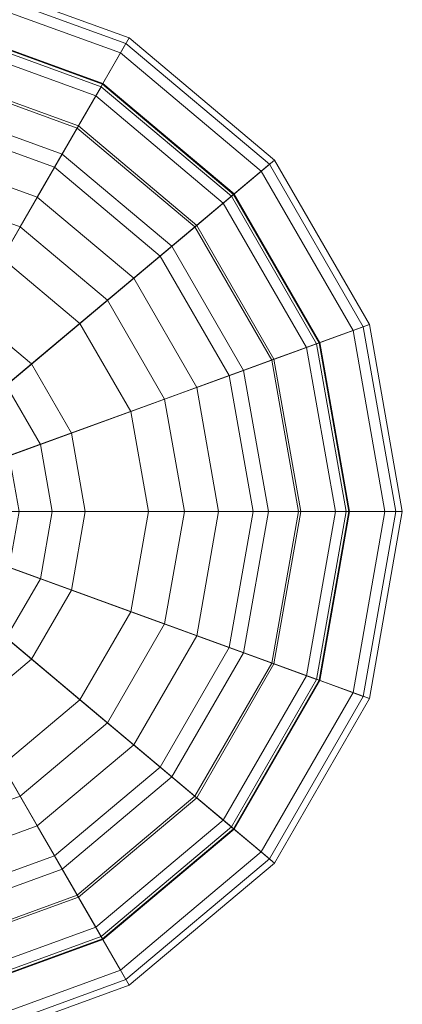
# Model space of a CAD drawing. Units: inches. Extents: x 375 to 1122, y 27 to 1069.
# Tile 43 of 155: x 719.669 to 720.617, y 297.867 to 300.305. Entities that reach past the tile are written whole.
import ezdxf

# ---------------------------------------------------------------- set-up
doc = ezdxf.new("R2010")
doc.units = ezdxf.units.IN
doc.layers.add('Furniture', color=30, linetype='Continuous', lineweight=18)

# ---------------------------------------------------------------- blocks, each defined once
blk = doc.blocks.new('A$C403C54AD')
for points in [[(1.180252, 0.891746, -0.031825), (1.180252, 0.857884, -0.028747), (1.180252, 0.857884, -0.028747), (1.16867, 0.889704, -0.031825)], [(1.180252, 0.88848, -0.028594), (1.180252, 0.891746, -0.031825), (1.16867, 0.889704, -0.031825), (1.169787, 0.886635, -0.028594)], [(1.191834, 0.889704, -0.031825), (1.180252, 0.857884, -0.028747), (1.180252, 0.857884, -0.028747), (1.180252, 0.891746, -0.031825)], [(1.190717, 0.886635, -0.028594), (1.191834, 0.889704, -0.031825), (1.180252, 0.891746, -0.031825), (1.180252, 0.88848, -0.028594)], [(1.180252, 0.88844, 0.131159), (1.180252, 0.891347, 0.117935), (1.168807, 0.889329, 0.117935), (1.169801, 0.886597, 0.131159)], [(1.180252, 0.891347, 0.117935), (1.180252, 0.890672, 0.089693), (1.169038, 0.888695, 0.089693), (1.168807, 0.889329, 0.117935)], [(1.190703, 0.886597, 0.131159), (1.191697, 0.889329, 0.117935), (1.180252, 0.891347, 0.117935), (1.180252, 0.88844, 0.131159)], [(1.191697, 0.889329, 0.117935), (1.191466, 0.888695, 0.089693), (1.180252, 0.890672, 0.089693), (1.180252, 0.891347, 0.117935)], [(1.180252, 0.890672, 0.089693), (1.180252, 0.885308, 0.071684), (1.170873, 0.883654, 0.071684), (1.169038, 0.888695, 0.089693)], [(1.191466, 0.888695, 0.089693), (1.189632, 0.883654, 0.071684), (1.180252, 0.885308, 0.071684), (1.180252, 0.890672, 0.089693)], [(1.169787, 0.886635, -0.028594), (1.16867, 0.889704, -0.031825), (1.158486, 0.883824, -0.031825), (1.160585, 0.881322, -0.028594)], [(1.16867, 0.889704, -0.031825), (1.180252, 0.857884, -0.028747), (1.180252, 0.857884, -0.028747), (1.158486, 0.883824, -0.031825)], [(1.202018, 0.883824, -0.031825), (1.180252, 0.857884, -0.028747), (1.180252, 0.857884, -0.028747), (1.191834, 0.889704, -0.031825)], [(1.199919, 0.881322, -0.028594), (1.202018, 0.883824, -0.031825), (1.191834, 0.889704, -0.031825), (1.190717, 0.886635, -0.028594)], [(1.169801, 0.886597, 0.131159), (1.168807, 0.889329, 0.117935), (1.158742, 0.883518, 0.117935), (1.160611, 0.881291, 0.131159)], [(1.168807, 0.889329, 0.117935), (1.169038, 0.888695, 0.089693), (1.159176, 0.883001, 0.089693), (1.158742, 0.883518, 0.117935)], [(1.199893, 0.881291, 0.131159), (1.201762, 0.883518, 0.117935), (1.191697, 0.889329, 0.117935), (1.190703, 0.886597, 0.131159)], [(1.201762, 0.883518, 0.117935), (1.201328, 0.883001, 0.089693), (1.191466, 0.888695, 0.089693), (1.191697, 0.889329, 0.117935)], [(1.169038, 0.888695, 0.089693), (1.170873, 0.883654, 0.071684), (1.162624, 0.878892, 0.071684), (1.159176, 0.883001, 0.089693)], [(1.180252, 0.872098, -0.02532), (1.180252, 0.88848, -0.028594), (1.169787, 0.886635, -0.028594), (1.17539, 0.871241, -0.02532)], [(1.180252, 0.883444, 0.140564), (1.180252, 0.88844, 0.131159), (1.169801, 0.886597, 0.131159), (1.17151, 0.881902, 0.140564)], [(1.185114, 0.871241, -0.02532), (1.190717, 0.886635, -0.028594), (1.180252, 0.88848, -0.028594), (1.180252, 0.872098, -0.02532)], [(1.188994, 0.881902, 0.140564), (1.190703, 0.886597, 0.131159), (1.180252, 0.88844, 0.131159), (1.180252, 0.883444, 0.140564)], [(1.201328, 0.883001, 0.089693), (1.19788, 0.878892, 0.071684), (1.189632, 0.883654, 0.071684), (1.191466, 0.888695, 0.089693)], [(1.180252, 0.888263, 0.117718), (1.180252, 0.885453, 0.130354), (1.170823, 0.88379, 0.130354), (1.169862, 0.886431, 0.117718)], [(1.180252, 0.887605, 0.090178), (1.180252, 0.888263, 0.117718), (1.169862, 0.886431, 0.117718), (1.170087, 0.885812, 0.090178)], [(1.190642, 0.886431, 0.117718), (1.189681, 0.88379, 0.130354), (1.180252, 0.885453, 0.130354), (1.180252, 0.888263, 0.117718)], [(1.190417, 0.885812, 0.090178), (1.190642, 0.886431, 0.117718), (1.180252, 0.888263, 0.117718), (1.180252, 0.887605, 0.090178)], [(1.180252, 0.882497, 0.073031), (1.180252, 0.887605, 0.090178), (1.170087, 0.885812, 0.090178), (1.171834, 0.881013, 0.073031)], [(1.18867, 0.881013, 0.073031), (1.190417, 0.885812, 0.090178), (1.180252, 0.887605, 0.090178), (1.180252, 0.882497, 0.073031)], [(1.17539, 0.871241, -0.02532), (1.169787, 0.886635, -0.028594), (1.160585, 0.881322, -0.028594), (1.171115, 0.868773, -0.02532)], [(1.17151, 0.881902, 0.140564), (1.169801, 0.886597, 0.131159), (1.160611, 0.881291, 0.131159), (1.163823, 0.877464, 0.140564)], [(1.189389, 0.868773, -0.02532), (1.199919, 0.881322, -0.028594), (1.190717, 0.886635, -0.028594), (1.185114, 0.871241, -0.02532)], [(1.196681, 0.877464, 0.140564), (1.199893, 0.881291, 0.131159), (1.190703, 0.886597, 0.131159), (1.188994, 0.881902, 0.140564)], [(1.169862, 0.886431, 0.117718), (1.170823, 0.88379, 0.130354), (1.162531, 0.879003, 0.130354), (1.160725, 0.881156, 0.117718)], [(1.170087, 0.885812, 0.090178), (1.169862, 0.886431, 0.117718), (1.160725, 0.881156, 0.117718), (1.161148, 0.880651, 0.090178)], [(1.199779, 0.881156, 0.117718), (1.197973, 0.879003, 0.130354), (1.189681, 0.88379, 0.130354), (1.190642, 0.886431, 0.117718)], [(1.199356, 0.880651, 0.090178), (1.199779, 0.881156, 0.117718), (1.190642, 0.886431, 0.117718), (1.190417, 0.885812, 0.090178)], [(1.171834, 0.881013, 0.073031), (1.170087, 0.885812, 0.090178), (1.161148, 0.880651, 0.090178), (1.164431, 0.876739, 0.073031)], [(1.180252, 0.885453, 0.130354), (1.180252, 0.880365, 0.140564), (1.172563, 0.879009, 0.140564), (1.170823, 0.88379, 0.130354)], [(1.180252, 0.885308, 0.071684), (1.180252, 0.878242, 0.061451), (1.173289, 0.877014, 0.061451), (1.170873, 0.883654, 0.071684)], [(1.189681, 0.88379, 0.130354), (1.187941, 0.879009, 0.140564), (1.180252, 0.880365, 0.140564), (1.180252, 0.885453, 0.130354)], [(1.189632, 0.883654, 0.071684), (1.187215, 0.877014, 0.061451), (1.180252, 0.878242, 0.061451), (1.180252, 0.885308, 0.071684)], [(1.196073, 0.876739, 0.073031), (1.199356, 0.880651, 0.090178), (1.190417, 0.885812, 0.090178), (1.18867, 0.881013, 0.073031)], [(1.160585, 0.881322, -0.028594), (1.158486, 0.883824, -0.031825), (1.150927, 0.874815, -0.031825), (1.153755, 0.873182, -0.028594)], [(1.158486, 0.883824, -0.031825), (1.180252, 0.857884, -0.028747), (1.180252, 0.857884, -0.028747), (1.150927, 0.874815, -0.031825)], [(1.160611, 0.881291, 0.131159), (1.158742, 0.883518, 0.117935), (1.151272, 0.874616, 0.117935), (1.15379, 0.873162, 0.131159)], [(1.158742, 0.883518, 0.117935), (1.159176, 0.883001, 0.089693), (1.151856, 0.874278, 0.089693), (1.151272, 0.874616, 0.117935)], [(1.170823, 0.88379, 0.130354), (1.172563, 0.879009, 0.140564), (1.165801, 0.875106, 0.140564), (1.162531, 0.879003, 0.130354)], [(1.170873, 0.883654, 0.071684), (1.173289, 0.877014, 0.061451), (1.167166, 0.873479, 0.061451), (1.162624, 0.878892, 0.071684)], [(1.209578, 0.874815, -0.031825), (1.180252, 0.857884, -0.028747), (1.180252, 0.857884, -0.028747), (1.202018, 0.883824, -0.031825)], [(1.19788, 0.878892, 0.071684), (1.193338, 0.873479, 0.061451), (1.187215, 0.877014, 0.061451), (1.189632, 0.883654, 0.071684)], [(1.197973, 0.879003, 0.130354), (1.194703, 0.875106, 0.140564), (1.187941, 0.879009, 0.140564), (1.189681, 0.88379, 0.130354)], [(1.206714, 0.873162, 0.131159), (1.209232, 0.874616, 0.117935), (1.201762, 0.883518, 0.117935), (1.199893, 0.881291, 0.131159)], [(1.206749, 0.873182, -0.028594), (1.209578, 0.874815, -0.031825), (1.202018, 0.883824, -0.031825), (1.199919, 0.881322, -0.028594)], [(1.209232, 0.874616, 0.117935), (1.208648, 0.874278, 0.089693), (1.201328, 0.883001, 0.089693), (1.201762, 0.883518, 0.117935)], [(1.159176, 0.883001, 0.089693), (1.162624, 0.878892, 0.071684), (1.156502, 0.871596, 0.071684), (1.151856, 0.874278, 0.089693)], [(1.180252, 0.880365, 0.140564), (1.180252, 0.883444, 0.140564), (1.17151, 0.881902, 0.140564), (1.172563, 0.879009, 0.140564)], [(1.187941, 0.879009, 0.140564), (1.188994, 0.881902, 0.140564), (1.180252, 0.883444, 0.140564), (1.180252, 0.880365, 0.140564)], [(1.208648, 0.874278, 0.089693), (1.204002, 0.871596, 0.071684), (1.19788, 0.878892, 0.071684), (1.201328, 0.883001, 0.089693)], [(1.180252, 0.876011, 0.063639), (1.180252, 0.882497, 0.073031), (1.171834, 0.881013, 0.073031), (1.174052, 0.874918, 0.063639)], [(1.186452, 0.874918, 0.063639), (1.18867, 0.881013, 0.073031), (1.180252, 0.882497, 0.073031), (1.180252, 0.876011, 0.063639)], [(1.172563, 0.879009, 0.140564), (1.17151, 0.881902, 0.140564), (1.163823, 0.877464, 0.140564), (1.165801, 0.875106, 0.140564)], [(1.194703, 0.875106, 0.140564), (1.196681, 0.877464, 0.140564), (1.188994, 0.881902, 0.140564), (1.187941, 0.879009, 0.140564)], [(1.171115, 0.868773, -0.02532), (1.160585, 0.881322, -0.028594), (1.153755, 0.873182, -0.028594), (1.167942, 0.864991, -0.02532)], [(1.163823, 0.877464, 0.140564), (1.160611, 0.881291, 0.131159), (1.15379, 0.873162, 0.131159), (1.158117, 0.870664, 0.140564)], [(1.160725, 0.881156, 0.117718), (1.162531, 0.879003, 0.130354), (1.156376, 0.871669, 0.130354), (1.153943, 0.873073, 0.117718)], [(1.161148, 0.880651, 0.090178), (1.160725, 0.881156, 0.117718), (1.153943, 0.873073, 0.117718), (1.154513, 0.872744, 0.090178)], [(1.192562, 0.864991, -0.02532), (1.206749, 0.873182, -0.028594), (1.199919, 0.881322, -0.028594), (1.189389, 0.868773, -0.02532)], [(1.202387, 0.870664, 0.140564), (1.206714, 0.873162, 0.131159), (1.199893, 0.881291, 0.131159), (1.196681, 0.877464, 0.140564)], [(1.206561, 0.873073, 0.117718), (1.204128, 0.871669, 0.130354), (1.197973, 0.879003, 0.130354), (1.199779, 0.881156, 0.117718)], [(1.205991, 0.872744, 0.090178), (1.206561, 0.873073, 0.117718), (1.199779, 0.881156, 0.117718), (1.199356, 0.880651, 0.090178)], [(1.164431, 0.876739, 0.073031), (1.161148, 0.880651, 0.090178), (1.154513, 0.872744, 0.090178), (1.158936, 0.87019, 0.073031)], [(1.174052, 0.874918, 0.063639), (1.171834, 0.881013, 0.073031), (1.164431, 0.876739, 0.073031), (1.1686, 0.87177, 0.063639)], [(1.191904, 0.87177, 0.063639), (1.196073, 0.876739, 0.073031), (1.18867, 0.881013, 0.073031), (1.186452, 0.874918, 0.063639)], [(1.201568, 0.87019, 0.073031), (1.205991, 0.872744, 0.090178), (1.199356, 0.880651, 0.090178), (1.196073, 0.876739, 0.073031)], [(1.162531, 0.879003, 0.130354), (1.165801, 0.875106, 0.140564), (1.160783, 0.869125, 0.140564), (1.156376, 0.871669, 0.130354)], [(1.162624, 0.878892, 0.071684), (1.167166, 0.873479, 0.061451), (1.162622, 0.868063, 0.061451), (1.156502, 0.871596, 0.071684)], [(1.204002, 0.871596, 0.071684), (1.197882, 0.868063, 0.061451), (1.193338, 0.873479, 0.061451), (1.19788, 0.878892, 0.071684)], [(1.204128, 0.871669, 0.130354), (1.199721, 0.869125, 0.140564), (1.194703, 0.875106, 0.140564), (1.197973, 0.879003, 0.130354)], [(1.180252, 0.878242, 0.061451), (1.180252, 0.868003, 0.054084), (1.176791, 0.867392, 0.054084), (1.173289, 0.877014, 0.061451)], [(1.187215, 0.877014, 0.061451), (1.183713, 0.867392, 0.054084), (1.180252, 0.868003, 0.054084), (1.180252, 0.878242, 0.061451)], [(1.165801, 0.875106, 0.140564), (1.163823, 0.877464, 0.140564), (1.158117, 0.870664, 0.140564), (1.160783, 0.869125, 0.140564)], [(1.199721, 0.869125, 0.140564), (1.202387, 0.870664, 0.140564), (1.196681, 0.877464, 0.140564), (1.194703, 0.875106, 0.140564)], [(1.173289, 0.877014, 0.061451), (1.176791, 0.867392, 0.054084), (1.173748, 0.865635, 0.054084), (1.167166, 0.873479, 0.061451)], [(1.193338, 0.873479, 0.061451), (1.186756, 0.865635, 0.054084), (1.183713, 0.867392, 0.054084), (1.187215, 0.877014, 0.061451)], [(1.1686, 0.87177, 0.063639), (1.164431, 0.876739, 0.073031), (1.158936, 0.87019, 0.073031), (1.164553, 0.866948, 0.063639)], [(1.195951, 0.866948, 0.063639), (1.201568, 0.87019, 0.073031), (1.196073, 0.876739, 0.073031), (1.191904, 0.87177, 0.063639)], [(1.180252, 0.866788, 0.057003), (1.180252, 0.876011, 0.063639), (1.174052, 0.874918, 0.063639), (1.177207, 0.866251, 0.057003)], [(1.183297, 0.866251, 0.057003), (1.186452, 0.874918, 0.063639), (1.180252, 0.876011, 0.063639), (1.180252, 0.866788, 0.057003)], [(1.177207, 0.866251, 0.057003), (1.174052, 0.874918, 0.063639), (1.1686, 0.87177, 0.063639), (1.174529, 0.864705, 0.057003)], [(1.185975, 0.864705, 0.057003), (1.191904, 0.87177, 0.063639), (1.186452, 0.874918, 0.063639), (1.183297, 0.866251, 0.057003)], [(1.153755, 0.873182, -0.028594), (1.150927, 0.874815, -0.031825), (1.146904, 0.863764, -0.031825), (1.15012, 0.863197, -0.028594)], [(1.150927, 0.874815, -0.031825), (1.180252, 0.857884, -0.028747), (1.180252, 0.857884, -0.028747), (1.146904, 0.863764, -0.031825)], [(1.15379, 0.873162, 0.131159), (1.151272, 0.874616, 0.117935), (1.147297, 0.863695, 0.117935), (1.15016, 0.86319, 0.131159)], [(1.151272, 0.874616, 0.117935), (1.151856, 0.874278, 0.089693), (1.147962, 0.863578, 0.089693), (1.147297, 0.863695, 0.117935)], [(1.2136, 0.863764, -0.031825), (1.180252, 0.857884, -0.028747), (1.180252, 0.857884, -0.028747), (1.209578, 0.874815, -0.031825)], [(1.210344, 0.86319, 0.131159), (1.213207, 0.863695, 0.117935), (1.209232, 0.874616, 0.117935), (1.206714, 0.873162, 0.131159)], [(1.210384, 0.863197, -0.028594), (1.2136, 0.863764, -0.031825), (1.209578, 0.874815, -0.031825), (1.206749, 0.873182, -0.028594)], [(1.213207, 0.863695, 0.117935), (1.212542, 0.863578, 0.089693), (1.208648, 0.874278, 0.089693), (1.209232, 0.874616, 0.117935)], [(1.151856, 0.874278, 0.089693), (1.156502, 0.871596, 0.071684), (1.153245, 0.862646, 0.071684), (1.147962, 0.863578, 0.089693)], [(1.212542, 0.863578, 0.089693), (1.207259, 0.862646, 0.071684), (1.204002, 0.871596, 0.071684), (1.208648, 0.874278, 0.089693)], [(1.167942, 0.864991, -0.02532), (1.153755, 0.873182, -0.028594), (1.15012, 0.863197, -0.028594), (1.166254, 0.860352, -0.02532)], [(1.158117, 0.870664, 0.140564), (1.15379, 0.873162, 0.131159), (1.15016, 0.86319, 0.131159), (1.155081, 0.862322, 0.140564)], [(1.167166, 0.873479, 0.061451), (1.173748, 0.865635, 0.054084), (1.171489, 0.862943, 0.054084), (1.162622, 0.868063, 0.061451)], [(1.197882, 0.868063, 0.061451), (1.189015, 0.862943, 0.054084), (1.186756, 0.865635, 0.054084), (1.193338, 0.873479, 0.061451)], [(1.19425, 0.860352, -0.02532), (1.210384, 0.863197, -0.028594), (1.206749, 0.873182, -0.028594), (1.192562, 0.864991, -0.02532)], [(1.205423, 0.862322, 0.140564), (1.210344, 0.86319, 0.131159), (1.206714, 0.873162, 0.131159), (1.202387, 0.870664, 0.140564)], [(1.153943, 0.873073, 0.117718), (1.156376, 0.871669, 0.130354), (1.153102, 0.862671, 0.130354), (1.150335, 0.863159, 0.117718)], [(1.154513, 0.872744, 0.090178), (1.153943, 0.873073, 0.117718), (1.150335, 0.863159, 0.117718), (1.150983, 0.863045, 0.090178)], [(1.158936, 0.87019, 0.073031), (1.154513, 0.872744, 0.090178), (1.150983, 0.863045, 0.090178), (1.156013, 0.862158, 0.073031)], [(1.204491, 0.862158, 0.073031), (1.209521, 0.863045, 0.090178), (1.205991, 0.872744, 0.090178), (1.201568, 0.87019, 0.073031)], [(1.210169, 0.863159, 0.117718), (1.207402, 0.862671, 0.130354), (1.204128, 0.871669, 0.130354), (1.206561, 0.873073, 0.117718)], [(1.209521, 0.863045, 0.090178), (1.210169, 0.863159, 0.117718), (1.206561, 0.873073, 0.117718), (1.205991, 0.872744, 0.090178)], [(1.180252, 0.87005, -0.022455), (1.180252, 0.872098, -0.02532), (1.17539, 0.871241, -0.02532), (1.176091, 0.869317, -0.022455)], [(1.184413, 0.869317, -0.022455), (1.185114, 0.871241, -0.02532), (1.180252, 0.872098, -0.02532), (1.180252, 0.87005, -0.022455)], [(1.156376, 0.871669, 0.130354), (1.160783, 0.869125, 0.140564), (1.158112, 0.861788, 0.140564), (1.153102, 0.862671, 0.130354)], [(1.156502, 0.871596, 0.071684), (1.162622, 0.868063, 0.061451), (1.160204, 0.861419, 0.061451), (1.153245, 0.862646, 0.071684)], [(1.174529, 0.864705, 0.057003), (1.1686, 0.87177, 0.063639), (1.164553, 0.866948, 0.063639), (1.172541, 0.862336, 0.057003)], [(1.187963, 0.862336, 0.057003), (1.195951, 0.866948, 0.063639), (1.191904, 0.87177, 0.063639), (1.185975, 0.864705, 0.057003)], [(1.207259, 0.862646, 0.071684), (1.2003, 0.861419, 0.061451), (1.197882, 0.868063, 0.061451), (1.204002, 0.871596, 0.071684)], [(1.207402, 0.862671, 0.130354), (1.202392, 0.861788, 0.140564), (1.199721, 0.869125, 0.140564), (1.204128, 0.871669, 0.130354)], [(1.160783, 0.869125, 0.140564), (1.158117, 0.870664, 0.140564), (1.155081, 0.862322, 0.140564), (1.158112, 0.861788, 0.140564)], [(1.176091, 0.869317, -0.022455), (1.17539, 0.871241, -0.02532), (1.171115, 0.868773, -0.02532), (1.172432, 0.867204, -0.022455)], [(1.188073, 0.867204, -0.022455), (1.189389, 0.868773, -0.02532), (1.185114, 0.871241, -0.02532), (1.184413, 0.869317, -0.022455)], [(1.202392, 0.861788, 0.140564), (1.205423, 0.862322, 0.140564), (1.202387, 0.870664, 0.140564), (1.199721, 0.869125, 0.140564)], [(1.164553, 0.866948, 0.063639), (1.158936, 0.87019, 0.073031), (1.156013, 0.862158, 0.073031), (1.1624, 0.861032, 0.063639)], [(1.180252, 0.865955, -0.020408), (1.180252, 0.87005, -0.022455), (1.176091, 0.869317, -0.022455), (1.177492, 0.865468, -0.020408)], [(1.183012, 0.865468, -0.020408), (1.184413, 0.869317, -0.022455), (1.180252, 0.87005, -0.022455), (1.180252, 0.865955, -0.020408)], [(1.198104, 0.861032, 0.063639), (1.204491, 0.862158, 0.073031), (1.201568, 0.87019, 0.073031), (1.195951, 0.866948, 0.063639)], [(1.177492, 0.865468, -0.020408), (1.176091, 0.869317, -0.022455), (1.172432, 0.867204, -0.022455), (1.175064, 0.864067, -0.020408)], [(1.18544, 0.864067, -0.020408), (1.188073, 0.867204, -0.022455), (1.184413, 0.869317, -0.022455), (1.183012, 0.865468, -0.020408)], [(1.172432, 0.867204, -0.022455), (1.171115, 0.868773, -0.02532), (1.167942, 0.864991, -0.02532), (1.169716, 0.863967, -0.022455)], [(1.190789, 0.863967, -0.022455), (1.192562, 0.864991, -0.02532), (1.189389, 0.868773, -0.02532), (1.188073, 0.867204, -0.022455)], [(1.162622, 0.868063, 0.061451), (1.171489, 0.862943, 0.054084), (1.170287, 0.859641, 0.054084), (1.160204, 0.861419, 0.061451)], [(1.2003, 0.861419, 0.061451), (1.190217, 0.859641, 0.054084), (1.189015, 0.862943, 0.054084), (1.197882, 0.868063, 0.061451)]]:
    blk.add_3dface(points)

msp = doc.modelspace()

# ---------------------------------------------------------------- block references
at = {"layer": 'Furniture', "xscale": 39.9918517141215, "yscale": 39.9918517141215, "zscale": 39.9918517141215, "rotation": 270}
msp.add_blockref('A$C403C54AD', (684.9549, 346.2875, 0.024), dxfattribs=at)

doc.saveas('drawing.dxf')
